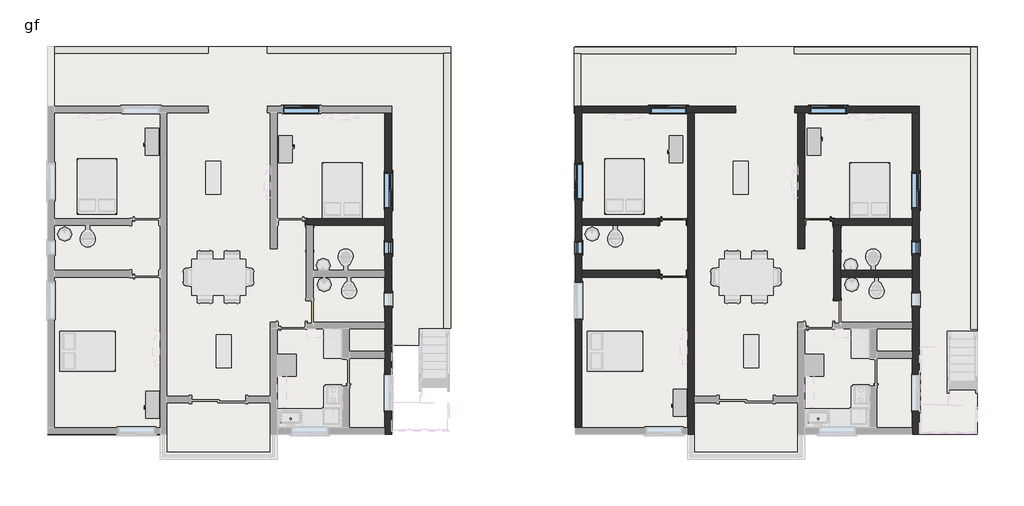
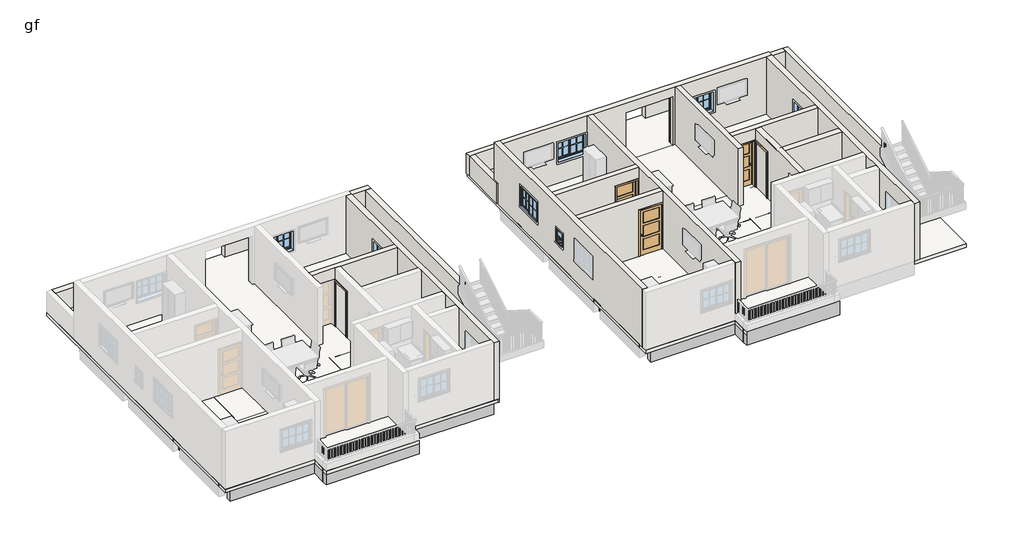
# One storey, part 2 of 8: 20 walls, 14 beams, 9 windows, 5 doors, 2 slabs.
"""IFC4 building model written with IfcOpenShell, lengths in millimetres."""

from ifc_helpers import new_model, si_unit, frame, origin, origin_with_axes, place, context, project, spatial, polyline, outline, extrude, faceted_brep, transform, mapped, element, save
from components import door_2334f446, door_80766924, door_85036156, window_608ea798, window_2eef0573, window_a5b1ea32

model = new_model("IFC4")

# Units and contexts
model_context = context("Model", 3, world=origin())
ifc_project = project(units=[si_unit("LENGTHUNIT", "METRE", prefix="MILLI")], contexts=[model_context])

# Site, building, storey
site = spatial("IfcSite", under=ifc_project)
building = spatial("IfcBuilding", under=site)
storey = spatial("IfcBuildingStorey", under=building, Name="gf", Elevation=609.6)

# Beams
placement = place(None, origin())
element("IfcBeam", 1, ObjectType="Concrete-Rectangular Beam", at=placement, inside=storey, context=model_context, shape_type="SweptSolid", body=[
    extrude(outline(polyline([(-16071.9993763, -4605.3064015), (-16071.9993763, -4376.7064015), (-12490.5993763, -4376.7064015), (-12490.5993763, -4605.3064015), (-16071.9993763, -4605.3064015)])), origin_with_axes(), (0.0, 0.0, 1.0), 609.6),
])
element("IfcBeam", 2, ObjectType="Concrete-Rectangular Beam", at=placement, inside=storey, context=model_context, shape_type="Brep", body=[
    faceted_brep([(-8528.1993763, -5443.5064015, 609.6), (-8528.1993763, -5214.9064015, 609.6), (-8756.7993763, -5214.9064015, 609.6), (-12261.9993763, -5214.9064015, 609.6), (-12490.5993763, -5214.9064015, 609.6), (-12490.5993763, -5443.5064015, 609.6), (-8528.1993763, -5443.5064015, 0.0), (-12490.5993763, -5443.5064015, 0.0), (-8528.1993763, -5214.9064015, 0.0), (-12490.5993763, -5214.9064015, 0.0), (-12261.9993763, -5214.9064015, 0.0), (-8756.7993763, -5214.9064015, 0.0)], [[[0, 1, 2, 3, 4, 5]], [[6, 0, 5, 7]], [[8, 6, 7, 9, 10, 11]], [[1, 8, 11, 10, 9, 4, 3, 2]], [[1, 0, 6, 8]], [[5, 4, 9, 7]]]),
])
element("IfcBeam", 3, ObjectType="Concrete-Rectangular Beam", at=placement, inside=storey, context=model_context, shape_type="Brep", body=[
    faceted_brep([(-8528.1993763, -4376.7064015, 609.6), (-8528.1993763, -4605.3064015, 609.6), (-4870.5993763, -4605.3064015, 609.6), (-4870.5993763, -4376.7064015, 609.6), (-6089.7993763, -4376.7064015, 609.6), (-6318.3993763, -4376.7064015, 609.6), (-8528.1993763, -4376.7064015, 0.0), (-4870.5993763, -4376.7064015, 0.0), (-6089.7993763, -4376.7064015, 0.0), (-6318.3993763, -4376.7064015, 0.0), (-8528.1993763, -4605.3064015, 0.0), (-4870.5993763, -4605.3064015, 0.0)], [[[0, 1, 2, 3, 4, 5]], [[6, 0, 5, 4, 3, 7, 8, 9]], [[10, 6, 9, 8, 7, 11]], [[1, 10, 11, 2]], [[1, 0, 6, 10]], [[3, 2, 11, 7]]]),
])
element("IfcBeam", 4, ObjectType="Concrete-Rectangular Beam", at=placement, inside=storey, context=model_context, shape_type="Brep", body=[
    faceted_brep([(-8528.1993763, -795.3064015, 609.6), (-8528.1993763, -1023.9064015, 609.6), (-6318.3993763, -1023.9064015, 609.6), (-6089.7993763, -1023.9064015, 609.6), (-4870.5993763, -1023.9064015, 609.6), (-4870.5993763, -795.3064015, 609.6), (-7308.9993763, -795.3064015, 609.6), (-7537.5993763, -795.3064015, 609.6), (-8528.1993763, -795.3064015, 0.0), (-4870.5993763, -795.3064015, 0.0), (-7308.9993763, -795.3064015, 0.0), (-7537.5993763, -795.3064015, 0.0), (-8528.1993763, -1023.9064015, 0.0), (-4870.5993763, -1023.9064015, 0.0), (-6089.7993763, -1023.9064015, 0.0), (-6318.3993763, -1023.9064015, 0.0)], [[[0, 1, 2, 3, 4, 5, 6, 7]], [[8, 0, 7, 6, 5, 9, 10, 11]], [[12, 8, 11, 10, 9, 13, 14, 15]], [[1, 12, 15, 14, 13, 4, 3, 2]], [[1, 0, 8, 12]], [[5, 4, 13, 9]]]),
])
element("IfcBeam", 5, ObjectType="Concrete-Rectangular Beam", at=placement, inside=storey, context=model_context, shape_type="Brep", body=[
    faceted_brep([(-6318.3993763, -4376.7064015, 609.6), (-6089.7993763, -4376.7064015, 609.6), (-6089.7993763, -2014.5064015, 609.6), (-6089.7993763, -1785.9064015, 609.6), (-6089.7993763, -1023.9064015, 609.6), (-6318.3993763, -1023.9064015, 609.6), (-6089.7993763, -4376.7064015, 0.0), (-6089.7993763, -2014.5064015, 0.0), (-6089.7993763, -1785.9064015, 0.0), (-6089.7993763, -1023.9064015, 0.0), (-6318.3993763, -4376.7064015, 0.0), (-6318.3993763, -1023.9064015, 0.0)], [[[0, 1, 2, 3, 4, 5]], [[1, 6, 7, 8, 9, 4, 3, 2]], [[6, 10, 11, 9, 8, 7]], [[10, 0, 5, 11]], [[1, 0, 10, 6]], [[5, 4, 9, 11]]]),
])
element("IfcBeam", 6, ObjectType="Concrete-Rectangular Beam", at=placement, inside=storey, context=model_context, shape_type="SweptSolid", body=[
    extrude(outline(polyline([(-4870.5993763, -1785.9064015), (-4870.5993763, -2014.5064015), (-6089.7993763, -2014.5064015), (-6089.7993763, -1785.9064015), (-4870.5993763, -1785.9064015)])), origin_with_axes(), (0.0, 0.0, 1.0), 609.6),
])
element("IfcBeam", 7, ObjectType="Concrete-Rectangular Beam", at=placement, inside=storey, context=model_context, shape_type="Brep", body=[
    faceted_brep([(-8756.7993763, -1023.9064015, 609.6), (-8756.7993763, -795.3064015, 609.6), (-12261.9993763, -795.3064015, 609.6), (-12261.9993763, -1023.9064015, 609.6), (-8756.7993763, -795.3064015, 0.0), (-12261.9993763, -795.3064015, 0.0), (-8756.7993763, -1023.9064015, 0.0), (-12261.9993763, -1023.9064015, 0.0)], [[[0, 1, 2, 3]], [[1, 4, 5, 2]], [[4, 6, 7, 5]], [[6, 0, 3, 7]], [[1, 0, 6, 4]], [[3, 2, 5, 7]]]),
    faceted_brep([(-16071.9993763, -1023.9064015, 609.6), (-16071.9993763, -795.3064015, 609.6), (-16071.9993763, -795.3064015, 0.0), (-16071.9993763, -1023.9064015, 0.0), (-12490.5993763, -795.3064015, 609.6), (-12490.5993763, -1023.9064015, 609.6), (-12490.5993763, -1023.9064015, 0.0), (-12490.5993763, -795.3064015, 0.0), (-13481.1993763, -795.3064015, 609.6), (-13709.7993763, -795.3064015, 609.6), (-13481.1993763, -795.3064015, 0.0), (-13709.7993763, -795.3064015, 0.0)], [[[0, 1, 2, 3]], [[4, 5, 6, 7]], [[1, 0, 5, 4, 8, 9]], [[2, 1, 9, 8, 4, 7, 10, 11]], [[3, 2, 11, 10, 7, 6]], [[0, 3, 6, 5]]]),
])
element("IfcBeam", 8, ObjectType="Concrete-Rectangular Beam", at=placement, inside=storey, context=model_context, shape_type="SweptSolid", body=[
    extrude(outline(polyline([(-12261.9993763, -3538.5064015), (-12261.9993763, -3309.9064015), (-8756.7993763, -3309.9064015), (-8756.7993763, -3538.5064015), (-12261.9993763, -3538.5064015)])), origin_with_axes(), (0.0, 0.0, 1.0), 609.6),
])
element("IfcBeam", 9, ObjectType="Concrete-Rectangular Beam", at=placement, inside=storey, context=model_context, shape_type="SweptSolid", body=[
    extrude(outline(polyline([(1802.5761273, -4605.3064015), (1802.5761273, -4376.7064015), (5383.9761273, -4376.7064015), (5383.9761273, -4605.3064015), (1802.5761273, -4605.3064015)])), origin_with_axes(), (0.0, 0.0, 1.0), 609.6),
])
element("IfcBeam", 10, ObjectType="Concrete-Rectangular Beam", at=placement, inside=storey, context=model_context, shape_type="Brep", body=[
    faceted_brep([(9346.3761273, -5443.5064015, 609.6), (9346.3761273, -5214.9064015, 609.6), (9117.7761273, -5214.9064015, 609.6), (5612.5761273, -5214.9064015, 609.6), (5383.9761273, -5214.9064015, 609.6), (5383.9761273, -5443.5064015, 609.6), (9346.3761273, -5443.5064015, 0.0), (5383.9761273, -5443.5064015, 0.0), (9346.3761273, -5214.9064015, 0.0), (5383.9761273, -5214.9064015, 0.0), (5612.5761273, -5214.9064015, 0.0), (9117.7761273, -5214.9064015, 0.0)], [[[0, 1, 2, 3, 4, 5]], [[6, 0, 5, 7]], [[8, 6, 7, 9, 10, 11]], [[1, 8, 11, 10, 9, 4, 3, 2]], [[1, 0, 6, 8]], [[5, 4, 9, 7]]]),
])
element("IfcBeam", 11, ObjectType="Concrete-Rectangular Beam", at=placement, inside=storey, context=model_context, shape_type="Brep", body=[
    faceted_brep([(9117.7761273, -1023.9064015, 609.6), (9117.7761273, -795.3064015, 609.6), (5612.5761273, -795.3064015, 609.6), (5612.5761273, -1023.9064015, 609.6), (9117.7761273, -795.3064015, 0.0), (5612.5761273, -795.3064015, 0.0), (9117.7761273, -1023.9064015, 0.0), (5612.5761273, -1023.9064015, 0.0)], [[[0, 1, 2, 3]], [[1, 4, 5, 2]], [[4, 6, 7, 5]], [[6, 0, 3, 7]], [[1, 0, 6, 4]], [[3, 2, 5, 7]]]),
    faceted_brep([(1802.5761273, -1023.9064015, 609.6), (1802.5761273, -795.3064015, 609.6), (1802.5761273, -795.3064015, 0.0), (1802.5761273, -1023.9064015, 0.0), (5383.9761273, -795.3064015, 609.6), (5383.9761273, -1023.9064015, 609.6), (5383.9761273, -1023.9064015, 0.0), (5383.9761273, -795.3064015, 0.0), (4393.3761273, -795.3064015, 609.6), (4164.7761273, -795.3064015, 609.6), (4393.3761273, -795.3064015, 0.0), (4164.7761273, -795.3064015, 0.0)], [[[0, 1, 2, 3]], [[4, 5, 6, 7]], [[1, 0, 5, 4, 8, 9]], [[2, 1, 9, 8, 4, 7, 10, 11]], [[3, 2, 11, 10, 7, 6]], [[0, 3, 6, 5]]]),
])
element("IfcBeam", 12, ObjectType="Concrete-Rectangular Beam", at=placement, inside=storey, context=model_context, shape_type="SweptSolid", body=[
    extrude(outline(polyline([(5612.5761273, -3538.5064015), (5612.5761273, -3309.9064015), (9117.7761273, -3309.9064015), (9117.7761273, -3538.5064015), (5612.5761273, -3538.5064015)])), origin_with_axes(), (0.0, 0.0, 1.0), 609.6),
])
element("IfcBeam", 13, ObjectType="Concrete-Rectangular Beam", at=placement, inside=storey, context=model_context, shape_type="SweptSolid", body=[
    extrude(outline(polyline([(-12490.5993763, -4605.3064015), (-12261.9993763, -4605.3064015), (-12261.9993763, -5214.9064015), (-12490.5993763, -5214.9064015), (-12490.5993763, -4605.3064015)])), origin_with_axes(), (0.0, 0.0, 1.0), 609.6),
])
element("IfcBeam", 14, ObjectType="Concrete-Rectangular Beam", at=placement, inside=storey, context=model_context, shape_type="SweptSolid", body=[
    extrude(outline(polyline([(5383.9761273, -4605.3064015), (5612.5761273, -4605.3064015), (5612.5761273, -5214.9064015), (5383.9761273, -5214.9064015), (5383.9761273, -4605.3064015)])), origin_with_axes(), (0.0, 0.0, 1.0), 609.6),
])

# Doors
door_shape = door_2334f446(model_context)
element("IfcDoor", 15, ObjectType="Door-Interior-Single-3_Panel_Vert-Wood : 36\" x 80\"", at=placement, inside=storey, context=model_context, shape_type="MappedRepresentation", body=[
    mapped(door_shape, transform((4888.6761273, 2598.7685985, 609.6), x_axis=(1.0, 0.0, 0.0), y_axis=(0.0, 1.0, 0.0), z_axis=(0.0, 0.0, 1.0))),
])
door_2_shape = door_80766924(model_context)
element("IfcDoor", 16, ObjectType="Door-Interior-Single-3_Panel_Vert-Wood : 36\" x 80\"", at=placement, inside=storey, context=model_context, shape_type="MappedRepresentation", body=[
    mapped(door_2_shape, transform((4888.6761273, 839.8185985, 609.6), x_axis=(1.0, 0.0, 0.0), y_axis=(0.0, 1.0, 0.0), z_axis=(0.0, 0.0, 1.0))),
])
element("IfcDoor", 17, ObjectType="Door-Interior-Single-3_Panel_Vert-Wood : 36\" x 80\"", at=placement, inside=storey, context=model_context, shape_type="MappedRepresentation", body=[
    mapped(door_2_shape, transform((9841.6761273, 2598.7685985, 609.6), x_axis=(-1.0, 0.0, 0.0), y_axis=(0.0, -1.0, 0.0), z_axis=(0.0, 0.0, 1.0))),
])
door_3_shape = door_85036156(model_context)
element("IfcDoor", 18, ObjectType="Single-Flush : 30\" x 80\"", at=placement, inside=storey, context=model_context, shape_type="MappedRepresentation", body=[
    mapped(door_3_shape, transform((-7423.2993763, 2024.0935985, 609.6), x_axis=(0.0, 1.0, 0.0), y_axis=(-1.0, 0.0, 0.0), z_axis=(0.0, 0.0, 1.0))),
])
element("IfcDoor", 19, ObjectType="Single-Flush : 30\" x 80\"", at=placement, inside=storey, context=model_context, shape_type="MappedRepresentation", body=[
    mapped(door_3_shape, transform((10451.2761273, 2024.0935985, 609.6), x_axis=(0.0, 1.0, 0.0), y_axis=(-1.0, 0.0, 0.0), z_axis=(0.0, 0.0, 1.0))),
])

# Slabs
element("IfcSlab", 20, at=placement, inside=storey, context=model_context, shape_type="SweptSolid", body=[
    extrude(outline(polyline([(15201.0761273, 8539.1935985), (15201.0761273, -4598.9564015), (9346.3761273, -4598.9564015), (9346.3761273, -5437.1564015), (5383.9761273, -5437.1564015), (5383.9761273, -4605.3064015), (1573.9761273, -4605.3064015), (1573.9761273, 8539.1935985), (15201.0761273, 8539.1935985)])), frame((0.0, 0.0, 457.2), z_axis=(0.0, 0.0, 1.0), x_axis=(1.0, 0.0, 0.0)), (0.0, 0.0, 1.0), 152.4),
])
element("IfcSlab", 21, at=placement, inside=storey, context=model_context, shape_type="SweptSolid", body=[
    extrude(outline(polyline([(-2647.3594779, 8539.1935985), (-2647.3594779, -998.5064015), (-3676.7993763, -998.5064015), (-3676.7993763, -1582.7064015), (-4641.9993763, -1582.7064015), (-4641.9993763, -4605.3064015), (-4692.7993763, -4605.3064015), (-8528.1993763, -4605.3064015), (-8528.1993763, -5443.5064015), (-12490.5993763, -5443.5064015), (-12490.5993763, -4611.6564015), (-16300.5993763, -4611.6564015), (-16300.5993763, 8539.1935985), (-2647.3594779, 8539.1935985)])), frame((0.0, 0.0, 457.2), z_axis=(0.0, 0.0, 1.0), x_axis=(1.0, 0.0, 0.0)), (0.0, 0.0, 1.0), 152.4),
])

# Walls
element("IfcWall", 22, at=placement, inside=storey, context=model_context, shape_type="Brep", body=[
    faceted_brep([(-4870.5993763, 6291.2935985, 609.6), (-4870.5993763, 2709.8935985, 609.6), (-4870.5993763, 2481.2935985, 609.6), (-4870.5993763, 957.2935985, 609.6), (-4870.5993763, 728.6935985, 609.6), (-4870.5993763, -795.3064015, 609.6), (-4870.5993763, -1023.9064015, 609.6), (-4870.5993763, -1785.9064015, 609.6), (-4870.5993763, -2014.5064015, 609.6), (-4870.5993763, -4376.7064015, 609.6), (-4870.5993763, -4605.3064015, 609.6), (-4870.5993763, -4605.3064015, 3200.4), (-4870.5993763, -4376.7064015, 3200.4), (-4870.5993763, -2014.5064015, 3200.4), (-4870.5993763, -1785.9064015, 3200.4), (-4870.5993763, -1023.9064015, 3200.4), (-4870.5993763, -795.3064015, 3200.4), (-4870.5993763, 728.6935985, 3200.4), (-4870.5993763, 957.2935985, 3200.4), (-4870.5993763, 2481.2935985, 3200.4), (-4870.5993763, 2709.8935985, 3200.4), (-4870.5993763, 6291.2935985, 3200.4), (-4870.5993763, 4271.9935985, 2438.4), (-4870.5993763, 3052.7935985, 2438.4), (-4870.5993763, 3052.7935985, 1524.0), (-4870.5993763, 4271.9935985, 1524.0), (-4870.5993763, -249.2064015, 2133.6), (-4870.5993763, -249.2064015, 1524.0), (-4870.5993763, 182.5935985, 1524.0), (-4870.5993763, 182.5935985, 2133.6), (-4870.5993763, 1503.3935985, 2133.6), (-4870.5993763, 1503.3935985, 1524.0), (-4870.5993763, 1935.1935985, 1524.0), (-4870.5993763, 1935.1935985, 2133.6), (-4870.5993763, -3805.2064015, 2438.4), (-4870.5993763, -3805.2064015, 1524.0), (-4870.5993763, -2586.0064015, 1524.0), (-4870.5993763, -2586.0064015, 2438.4), (-4641.9993763, 6291.2935985, 609.6), (-4641.9993763, 6291.2935985, 3200.4), (-4641.9993763, -4605.3064015, 3200.4), (-4641.9993763, -4605.3064015, 609.6), (-4641.9993763, 4271.9935985, 2438.4), (-4641.9993763, 4271.9935985, 1524.0), (-4641.9993763, 3052.7935985, 1524.0), (-4641.9993763, 3052.7935985, 2438.4), (-4641.9993763, -249.2064015, 2133.6), (-4641.9993763, 182.5935985, 2133.6), (-4641.9993763, 182.5935985, 1524.0), (-4641.9993763, -249.2064015, 1524.0), (-4641.9993763, 1503.3935985, 2133.6), (-4641.9993763, 1935.1935985, 2133.6), (-4641.9993763, 1935.1935985, 1524.0), (-4641.9993763, 1503.3935985, 1524.0), (-4641.9993763, -3805.2064015, 2438.4), (-4641.9993763, -2586.0064015, 2438.4), (-4641.9993763, -2586.0064015, 1524.0), (-4641.9993763, -3805.2064015, 1524.0)], [[[0, 1, 2, 3, 4, 5, 6, 7, 8, 9, 10, 11, 12, 13, 14, 15, 16, 17, 18, 19, 20, 21], [22, 23, 24, 25], [26, 27, 28, 29], [30, 31, 32, 33], [34, 35, 36, 37]], [[38, 39, 40, 41], [42, 43, 44, 45], [46, 47, 48, 49], [50, 51, 52, 53], [54, 55, 56, 57]], [[10, 9, 8, 7, 6, 5, 4, 3, 2, 1, 0, 38, 41]], [[21, 20, 19, 18, 17, 16, 15, 14, 13, 12, 11, 40, 39]], [[0, 21, 39, 38]], [[11, 10, 41, 40]], [[43, 42, 22, 25]], [[44, 43, 25, 24]], [[45, 44, 24, 23]], [[42, 45, 23, 22]], [[27, 26, 46, 49]], [[28, 27, 49, 48]], [[29, 28, 48, 47]], [[26, 29, 47, 46]], [[31, 30, 50, 53]], [[32, 31, 53, 52]], [[33, 32, 52, 51]], [[30, 33, 51, 50]], [[35, 34, 54, 57]], [[36, 35, 57, 56]], [[37, 36, 56, 55]], [[34, 37, 55, 54]]]),
])
element("IfcWall", 23, at=placement, inside=storey, context=model_context, shape_type="Brep", body=[
    faceted_brep([(-4870.5993763, 2481.2935985, 3200.4), (-7308.9993763, 2481.2935985, 3200.4), (-7537.5993763, 2481.2935985, 3200.4), (-8528.1993763, 2481.2935985, 3200.4), (-8528.1993763, 2481.2935985, 609.6), (-8515.4993763, 2481.2935985, 609.6), (-8515.4993763, 2481.2935985, 2667.0), (-7550.2993763, 2481.2935985, 2667.0), (-7550.2993763, 2481.2935985, 609.6), (-7537.5993763, 2481.2935985, 609.6), (-7308.9993763, 2481.2935985, 609.6), (-4870.5993763, 2481.2935985, 609.6), (-8528.1993763, 2709.8935985, 3200.4), (-4870.5993763, 2709.8935985, 3200.4), (-4870.5993763, 2709.8935985, 609.6), (-7550.2993763, 2709.8935985, 609.6), (-7550.2993763, 2709.8935985, 2667.0), (-8515.4993763, 2709.8935985, 2667.0), (-8515.4993763, 2709.8935985, 609.6), (-8528.1993763, 2709.8935985, 609.6)], [[[0, 1, 2, 3, 4, 5, 6, 7, 8, 9, 10, 11]], [[12, 13, 14, 15, 16, 17, 18, 19]], [[14, 11, 10, 9, 8, 15]], [[4, 19, 18, 5]], [[3, 2, 1, 0, 13, 12]], [[0, 11, 14, 13]], [[17, 6, 5, 18]], [[6, 17, 16, 7]], [[7, 16, 15, 8]], [[4, 3, 12, 19]]]),
])
element("IfcWall", 24, at=placement, inside=storey, context=model_context, shape_type="Brep", body=[
    faceted_brep([(1573.9761273, 6519.8935985, 609.6), (1573.9761273, -4376.7064015, 609.6), (1573.9761273, -4376.7064015, 3200.4), (1573.9761273, 6519.8935985, 3200.4), (1573.9761273, 4576.7935985, 2438.4), (1573.9761273, 3357.5935985, 2438.4), (1573.9761273, 3357.5935985, 1524.0), (1573.9761273, 4576.7935985, 1524.0), (1573.9761273, -681.0064015, 2438.4), (1573.9761273, -681.0064015, 1524.0), (1573.9761273, 538.1935985, 1524.0), (1573.9761273, 538.1935985, 2438.4), (1573.9761273, 1935.1935985, 2133.6), (1573.9761273, 1503.3935985, 2133.6), (1573.9761273, 1503.3935985, 1524.0), (1573.9761273, 1935.1935985, 1524.0), (1802.5761273, 6519.8935985, 609.6), (1802.5761273, 6519.8935985, 3200.4), (1802.5761273, 6291.2935985, 3200.4), (1802.5761273, 2709.8935985, 3200.4), (1802.5761273, 2481.2935985, 3200.4), (1802.5761273, 957.2935985, 3200.4), (1802.5761273, 728.6935985, 3200.4), (1802.5761273, -4376.7064015, 3200.4), (1802.5761273, -4376.7064015, 609.6), (1802.5761273, 728.6935985, 609.6), (1802.5761273, 957.2935985, 609.6), (1802.5761273, 2481.2935985, 609.6), (1802.5761273, 2709.8935985, 609.6), (1802.5761273, 6291.2935985, 609.6), (1802.5761273, 4576.7935985, 2438.4), (1802.5761273, 4576.7935985, 1524.0), (1802.5761273, 3357.5935985, 1524.0), (1802.5761273, 3357.5935985, 2438.4), (1802.5761273, -681.0064015, 2438.4), (1802.5761273, 538.1935985, 2438.4), (1802.5761273, 538.1935985, 1524.0), (1802.5761273, -681.0064015, 1524.0), (1802.5761273, 1935.1935985, 2133.6), (1802.5761273, 1935.1935985, 1524.0), (1802.5761273, 1503.3935985, 1524.0), (1802.5761273, 1503.3935985, 2133.6)], [[[0, 1, 2, 3], [4, 5, 6, 7], [8, 9, 10, 11], [12, 13, 14, 15]], [[16, 17, 18, 19, 20, 21, 22, 23, 24, 25, 26, 27, 28, 29], [30, 31, 32, 33], [34, 35, 36, 37], [38, 39, 40, 41]], [[1, 0, 16, 29, 28, 27, 26, 25, 24]], [[3, 2, 23, 22, 21, 20, 19, 18, 17]], [[0, 3, 17, 16]], [[2, 1, 24, 23]], [[31, 30, 4, 7]], [[32, 31, 7, 6]], [[33, 32, 6, 5]], [[30, 33, 5, 4]], [[9, 8, 34, 37]], [[10, 9, 37, 36]], [[11, 10, 36, 35]], [[8, 11, 35, 34]], [[39, 38, 12, 15]], [[40, 39, 15, 14]], [[41, 40, 14, 13]], [[38, 41, 13, 12]]]),
])
element("IfcWall", 25, at=placement, inside=storey, context=model_context, shape_type="SweptSolid", body=[
    extrude(outline(polyline([(3200.4, 5383.9761273), (3200.4, 1802.5761273), (609.6, 1802.5761273), (609.6, 4406.0761273), (2667.0, 4406.0761273), (2667.0, 5371.2761273), (609.6, 5371.2761273), (609.6, 5383.9761273), (3200.4, 5383.9761273)])), frame((0.0, 2481.2935985, 0.0), z_axis=(0.0, 1.0, 0.0), x_axis=(0.0, 0.0, 1.0)), (0.0, 0.0, 1.0), 228.6),
])
element("IfcWall", 26, at=placement, inside=storey, context=model_context, shape_type="Brep", body=[
    faceted_brep([(13232.5761273, 6291.2935985, 3200.4), (13003.9761273, 6291.2935985, 3200.4), (9346.3761273, 6291.2935985, 3200.4), (9117.7761273, 6291.2935985, 3200.4), (5612.5761273, 6291.2935985, 3200.4), (5383.9761273, 6291.2935985, 3200.4), (1802.5761273, 6291.2935985, 3200.4), (1802.5761273, 6291.2935985, 609.6), (5383.9761273, 6291.2935985, 609.6), (5612.5761273, 6291.2935985, 609.6), (7012.8761273, 6291.2935985, 609.6), (7012.8761273, 6291.2935985, 2779.1), (9012.8761273, 6291.2935985, 2779.1), (9012.8761273, 6291.2935985, 609.6), (9117.7761273, 6291.2935985, 609.6), (9346.3761273, 6291.2935985, 609.6), (13003.9761273, 6291.2935985, 609.6), (13232.5761273, 6291.2935985, 609.6), (9536.8761273, 6291.2935985, 2438.4), (10756.0761273, 6291.2935985, 2438.4), (10756.0761273, 6291.2935985, 1524.0), (9536.8761273, 6291.2935985, 1524.0), (5345.8761273, 6291.2935985, 2438.4), (5345.8761273, 6291.2935985, 1524.0), (4126.6761273, 6291.2935985, 1524.0), (4126.6761273, 6291.2935985, 2438.4), (1802.5761273, 6519.8935985, 3200.4), (13232.5761273, 6519.8935985, 3200.4), (13232.5761273, 6519.8935985, 609.6), (9012.8761273, 6519.8935985, 609.6), (9012.8761273, 6519.8935985, 2779.1), (7012.8761273, 6519.8935985, 2779.1), (7012.8761273, 6519.8935985, 609.6), (1802.5761273, 6519.8935985, 609.6), (9536.8761273, 6519.8935985, 2438.4), (9536.8761273, 6519.8935985, 1524.0), (10756.0761273, 6519.8935985, 1524.0), (10756.0761273, 6519.8935985, 2438.4), (5345.8761273, 6519.8935985, 2438.4), (4126.6761273, 6519.8935985, 2438.4), (4126.6761273, 6519.8935985, 1524.0), (5345.8761273, 6519.8935985, 1524.0), (7012.8761273, 6499.8935985, 609.6), (6997.8761273, 6499.8935985, 609.6), (6997.8761273, 6429.8935985, 609.6), (7012.8761273, 6429.8935985, 609.6), (9012.8761273, 6429.8935985, 609.6), (9027.8761273, 6429.8935985, 609.6), (9027.8761273, 6499.8935985, 609.6), (9012.8761273, 6499.8935985, 609.6), (9012.8761273, 6499.8935985, 2779.1), (7012.8761273, 6499.8935985, 2779.1), (7012.8761273, 6429.8935985, 2779.1), (9012.8761273, 6429.8935985, 2779.1), (6997.8761273, 6429.8935985, 2794.1), (9027.8761273, 6429.8935985, 2794.1), (9027.8761273, 6499.8935985, 2794.1), (6997.8761273, 6499.8935985, 2794.1)], [[[0, 1, 2, 3, 4, 5, 6, 7, 8, 9, 10, 11, 12, 13, 14, 15, 16, 17], [18, 19, 20, 21], [22, 23, 24, 25]], [[26, 27, 28, 29, 30, 31, 32, 33], [34, 35, 36, 37], [38, 39, 40, 41]], [[7, 33, 32, 42, 43, 44, 45, 10, 9, 8]], [[28, 17, 16, 15, 14, 13, 46, 47, 48, 49, 29]], [[6, 5, 4, 3, 2, 1, 0, 27, 26]], [[7, 6, 26, 33]], [[0, 17, 28, 27]], [[50, 51, 31, 30]], [[52, 53, 12, 11]], [[45, 52, 11, 10]], [[53, 46, 13, 12]], [[53, 52, 45, 44, 54, 55, 47, 46]], [[47, 55, 56, 48]], [[51, 50, 49, 48, 56, 57, 43, 42]], [[49, 50, 30, 29]], [[51, 42, 32, 31]], [[54, 44, 43, 57]], [[55, 54, 57, 56]], [[35, 34, 18, 21]], [[36, 35, 21, 20]], [[37, 36, 20, 19]], [[34, 37, 19, 18]], [[23, 22, 38, 41]], [[24, 23, 41, 40]], [[25, 24, 40, 39]], [[22, 25, 39, 38]]]),
])
element("IfcWall", 27, at=placement, inside=storey, context=model_context, shape_type="Brep", body=[
    faceted_brep([(13003.9761273, 6291.2935985, 609.6), (13003.9761273, 2709.8935985, 609.6), (13003.9761273, 2481.2935985, 609.6), (13003.9761273, 957.2935985, 609.6), (13003.9761273, 728.6935985, 609.6), (13003.9761273, -795.3064015, 609.6), (13003.9761273, -1023.9064015, 609.6), (13003.9761273, -1785.9064015, 609.6), (13003.9761273, -2014.5064015, 609.6), (13003.9761273, -4376.7064015, 609.6), (13003.9761273, -4605.3064015, 609.6), (13003.9761273, -4605.3064015, 3200.4), (13003.9761273, -4376.7064015, 3200.4), (13003.9761273, -2014.5064015, 3200.4), (13003.9761273, -1785.9064015, 3200.4), (13003.9761273, -1023.9064015, 3200.4), (13003.9761273, -795.3064015, 3200.4), (13003.9761273, 728.6935985, 3200.4), (13003.9761273, 957.2935985, 3200.4), (13003.9761273, 2481.2935985, 3200.4), (13003.9761273, 2709.8935985, 3200.4), (13003.9761273, 6291.2935985, 3200.4), (13003.9761273, 4271.9935985, 2438.4), (13003.9761273, 3052.7935985, 2438.4), (13003.9761273, 3052.7935985, 1524.0), (13003.9761273, 4271.9935985, 1524.0), (13003.9761273, -249.2064015, 2133.6), (13003.9761273, -249.2064015, 1524.0), (13003.9761273, 182.5935985, 1524.0), (13003.9761273, 182.5935985, 2133.6), (13003.9761273, 1503.3935985, 2133.6), (13003.9761273, 1503.3935985, 1524.0), (13003.9761273, 1935.1935985, 1524.0), (13003.9761273, 1935.1935985, 2133.6), (13003.9761273, -3805.2064015, 2438.4), (13003.9761273, -3805.2064015, 1524.0), (13003.9761273, -2586.0064015, 1524.0), (13003.9761273, -2586.0064015, 2438.4), (13232.5761273, 6291.2935985, 609.6), (13232.5761273, 6291.2935985, 3200.4), (13232.5761273, -4605.3064015, 3200.4), (13232.5761273, -4605.3064015, 609.6), (13232.5761273, 4271.9935985, 2438.4), (13232.5761273, 4271.9935985, 1524.0), (13232.5761273, 3052.7935985, 1524.0), (13232.5761273, 3052.7935985, 2438.4), (13232.5761273, -249.2064015, 2133.6), (13232.5761273, 182.5935985, 2133.6), (13232.5761273, 182.5935985, 1524.0), (13232.5761273, -249.2064015, 1524.0), (13232.5761273, 1503.3935985, 2133.6), (13232.5761273, 1935.1935985, 2133.6), (13232.5761273, 1935.1935985, 1524.0), (13232.5761273, 1503.3935985, 1524.0), (13232.5761273, -3805.2064015, 2438.4), (13232.5761273, -2586.0064015, 2438.4), (13232.5761273, -2586.0064015, 1524.0), (13232.5761273, -3805.2064015, 1524.0)], [[[0, 1, 2, 3, 4, 5, 6, 7, 8, 9, 10, 11, 12, 13, 14, 15, 16, 17, 18, 19, 20, 21], [22, 23, 24, 25], [26, 27, 28, 29], [30, 31, 32, 33], [34, 35, 36, 37]], [[38, 39, 40, 41], [42, 43, 44, 45], [46, 47, 48, 49], [50, 51, 52, 53], [54, 55, 56, 57]], [[10, 9, 8, 7, 6, 5, 4, 3, 2, 1, 0, 38, 41]], [[21, 20, 19, 18, 17, 16, 15, 14, 13, 12, 11, 40, 39]], [[0, 21, 39, 38]], [[43, 42, 22, 25]], [[44, 43, 25, 24]], [[45, 44, 24, 23]], [[42, 45, 23, 22]], [[27, 26, 46, 49]], [[28, 27, 49, 48]], [[29, 28, 48, 47]], [[26, 29, 47, 46]], [[31, 30, 50, 53]], [[32, 31, 53, 52]], [[33, 32, 52, 51]], [[30, 33, 51, 50]], [[35, 34, 54, 57]], [[36, 35, 57, 56]], [[37, 36, 56, 55]], [[34, 37, 55, 54]], [[11, 10, 41, 40]]]),
])
element("IfcWall", 28, at=placement, inside=storey, context=model_context, shape_type="Brep", body=[
    faceted_brep([(9117.7761273, 6291.2935985, 609.6), (9117.7761273, 1681.1935985, 609.6), (9117.7761273, 1681.1935985, 3200.4), (9117.7761273, 6291.2935985, 3200.4), (9346.3761273, 6291.2935985, 609.6), (9346.3761273, 6291.2935985, 3200.4), (9346.3761273, 2709.8935985, 3200.4), (9346.3761273, 2481.2935985, 3200.4), (9346.3761273, 1681.1935985, 3200.4), (9346.3761273, 1681.1935985, 609.6), (9346.3761273, 2481.2935985, 609.6), (9346.3761273, 2709.8935985, 609.6)], [[[0, 1, 2, 3]], [[4, 5, 6, 7, 8, 9, 10, 11]], [[1, 0, 4, 11, 10, 9]], [[2, 1, 9, 8]], [[3, 2, 8, 7, 6, 5]], [[0, 3, 5, 4]]]),
])
element("IfcWall", 29, at=placement, inside=storey, context=model_context, shape_type="SweptSolid", body=[
    extrude(outline(polyline([(10565.5761273, 957.2935985), (13003.9761273, 957.2935985), (13003.9761273, 728.6935985), (10565.5761273, 728.6935985), (10565.5761273, 957.2935985)])), frame((0.0, 0.0, 609.6), z_axis=(0.0, 0.0, 1.0), x_axis=(1.0, 0.0, 0.0)), (0.0, 0.0, 1.0), 2590.8),
])
element("IfcWall", 30, at=placement, inside=storey, context=model_context, shape_type="Brep", body=[
    faceted_brep([(10565.5761273, 2481.2935985, 3200.4), (10565.5761273, 957.2935985, 3200.4), (10565.5761273, 728.6935985, 3200.4), (10565.5761273, -795.3064015, 3200.4), (10565.5761273, -795.3064015, 2641.6), (10565.5761273, -71.4064015, 2641.6), (10565.5761273, -71.4064015, 609.6), (10565.5761273, 728.6935985, 609.6), (10565.5761273, 957.2935985, 609.6), (10565.5761273, 2481.2935985, 609.6), (10336.9761273, -795.3064015, 3200.4), (10336.9761273, 2481.2935985, 3200.4), (10336.9761273, 2481.2935985, 609.6), (10336.9761273, -71.4064015, 609.6), (10336.9761273, -71.4064015, 2641.6), (10336.9761273, -795.3064015, 2641.6)], [[[0, 1, 2, 3, 4, 5, 6, 7, 8, 9]], [[10, 11, 12, 13, 14, 15]], [[12, 9, 8, 7, 6, 13]], [[3, 2, 1, 0, 11, 10]], [[3, 10, 15, 4]], [[0, 9, 12, 11]], [[14, 5, 4, 15]], [[5, 14, 13, 6]]]),
])
element("IfcWall", 31, at=placement, inside=storey, context=model_context, shape_type="SweptSolid", body=[
    extrude(outline(polyline([(2481.2935985, 609.6), (2405.0935985, 609.6), (2405.0935985, 2641.6), (1643.0935985, 2641.6), (1643.0935985, 609.6), (957.2935985, 609.6), (957.2935985, 3200.4), (2481.2935985, 3200.4), (2481.2935985, 609.6)])), frame((10336.9761273, 0.0, 0.0), z_axis=(1.0, 0.0, 0.0), x_axis=(0.0, 1.0, 0.0)), (0.0, 0.0, 1.0), 228.6),
])
element("IfcWall", 32, at=placement, inside=storey, context=model_context, shape_type="Brep", body=[
    faceted_brep([(13003.9761273, 2481.2935985, 3200.4), (10565.5761273, 2481.2935985, 3200.4), (10336.9761273, 2481.2935985, 3200.4), (9346.3761273, 2481.2935985, 3200.4), (9346.3761273, 2481.2935985, 609.6), (9359.0761273, 2481.2935985, 609.6), (9359.0761273, 2481.2935985, 2667.0), (10324.2761273, 2481.2935985, 2667.0), (10324.2761273, 2481.2935985, 609.6), (10336.9761273, 2481.2935985, 609.6), (10565.5761273, 2481.2935985, 609.6), (13003.9761273, 2481.2935985, 609.6), (9346.3761273, 2709.8935985, 3200.4), (13003.9761273, 2709.8935985, 3200.4), (13003.9761273, 2709.8935985, 609.6), (10324.2761273, 2709.8935985, 609.6), (10324.2761273, 2709.8935985, 2667.0), (9359.0761273, 2709.8935985, 2667.0), (9359.0761273, 2709.8935985, 609.6), (9346.3761273, 2709.8935985, 609.6)], [[[0, 1, 2, 3, 4, 5, 6, 7, 8, 9, 10, 11]], [[12, 13, 14, 15, 16, 17, 18, 19]], [[14, 11, 10, 9, 8, 15]], [[4, 19, 18, 5]], [[3, 2, 1, 0, 13, 12]], [[0, 11, 14, 13]], [[17, 6, 5, 18]], [[6, 17, 16, 7]], [[7, 16, 15, 8]], [[4, 3, 12, 19]]]),
])
element("IfcWall", 33, at=placement, inside=storey, context=model_context, shape_type="SweptSolid", body=[
    extrude(outline(polyline([(3200.4, 5383.9761273), (3200.4, 1802.5761273), (609.6, 1802.5761273), (609.6, 4406.0761273), (2667.0, 4406.0761273), (2667.0, 5371.2761273), (609.6, 5371.2761273), (609.6, 5383.9761273), (3200.4, 5383.9761273)])), frame((0.0, 728.6935985, 0.0), z_axis=(0.0, 1.0, 0.0), x_axis=(0.0, 0.0, 1.0)), (0.0, 0.0, 1.0), 228.6),
])
element("IfcWall", 34, at=placement, inside=storey, context=model_context, shape_type="Brep", body=[
    faceted_brep([(5612.5761273, -4605.3064015, 609.6), (5612.5761273, -3538.5064015, 609.6), (5612.5761273, -3309.9064015, 609.6), (5612.5761273, 6291.2935985, 609.6), (5612.5761273, 6291.2935985, 3200.4), (5612.5761273, -3309.9064015, 3200.4), (5612.5761273, -3538.5064015, 3200.4), (5612.5761273, -4605.3064015, 3200.4), (5383.9761273, -4605.3064015, 609.6), (5383.9761273, -4605.3064015, 3200.4), (5383.9761273, -4376.7064015, 3200.4), (5383.9761273, 728.6935985, 3200.4), (5383.9761273, 957.2935985, 3200.4), (5383.9761273, 2481.2935985, 3200.4), (5383.9761273, 2709.8935985, 3200.4), (5383.9761273, 6291.2935985, 3200.4), (5383.9761273, 6291.2935985, 609.6), (5383.9761273, 2709.8935985, 609.6), (5383.9761273, 2481.2935985, 609.6), (5383.9761273, 957.2935985, 609.6), (5383.9761273, 728.6935985, 609.6), (5383.9761273, -4376.7064015, 609.6)], [[[0, 1, 2, 3, 4, 5, 6, 7]], [[8, 9, 10, 11, 12, 13, 14, 15, 16, 17, 18, 19, 20, 21]], [[3, 2, 1, 0, 8, 21, 20, 19, 18, 17, 16]], [[7, 6, 5, 4, 15, 14, 13, 12, 11, 10, 9]], [[4, 3, 16, 15]], [[0, 7, 9, 8]]]),
])
element("IfcWall", 35, at=placement, inside=storey, context=model_context, shape_type="Brep", body=[
    faceted_brep([(15204.9910257, -1042.9564015, 609.6), (15204.9910257, 8523.3185985, 609.6), (15204.9910257, 8523.3185985, 1524.0), (15204.9910257, -1042.9564015, 1524.0), (14976.3910257, -1042.9564015, 609.6), (14976.3910257, -1042.9564015, 1524.0), (14976.3910257, 8294.7185985, 1524.0), (14976.3910257, 8523.3185985, 1524.0), (14976.3910257, 8523.3185985, 609.6), (14976.3910257, 8294.7185985, 609.6)], [[[0, 1, 2, 3]], [[4, 5, 6, 7, 8, 9]], [[1, 0, 4, 9, 8]], [[3, 2, 7, 6, 5]], [[0, 3, 5, 4]], [[2, 1, 8, 7]]]),
])
element("IfcWall", 36, at=placement, inside=storey, context=model_context, shape_type="SweptSolid", body=[
    extrude(outline(polyline([(9003.4761273, 8523.3185985), (14976.3910257, 8523.3185985), (14976.3910257, 8294.7185985), (9003.4761273, 8294.7185985), (9003.4761273, 8523.3185985)])), frame((0.0, 0.0, 609.6), z_axis=(0.0, 0.0, 1.0), x_axis=(1.0, 0.0, 0.0)), (0.0, 0.0, 1.0), 914.4),
])
element("IfcWall", 37, at=placement, inside=storey, context=model_context, shape_type="SweptSolid", body=[
    extrude(outline(polyline([(1539.7910257, 6275.4185985), (1539.7910257, 8294.7185985), (1768.3910257, 8294.7185985), (1768.3910257, 6275.4185985), (1539.7910257, 6275.4185985)])), frame((0.0, 0.0, 609.6), z_axis=(0.0, 0.0, 1.0), x_axis=(1.0, 0.0, 0.0)), (0.0, 0.0, 1.0), 914.4),
])
element("IfcWall", 38, at=placement, inside=storey, context=model_context, shape_type="SweptSolid", body=[
    extrude(outline(polyline([(-10852.2993763, 8310.5935985), (-16071.9993763, 8310.5935985), (-16071.9993763, 8539.1935985), (-10852.2993763, 8539.1935985), (-10852.2993763, 8310.5935985)])), frame((0.0, 0.0, 609.6), z_axis=(0.0, 0.0, 1.0), x_axis=(1.0, 0.0, 0.0)), (0.0, 0.0, 1.0), 914.4),
])
element("IfcWall", 39, at=placement, inside=storey, context=model_context, shape_type="SweptSolid", body=[
    extrude(outline(polyline([(-2875.9594779, -998.5064015), (-2875.9594779, 8310.5935985), (-2647.3594779, 8310.5935985), (-2647.3594779, -998.5064015), (-2875.9594779, -998.5064015)])), frame((0.0, 0.0, 609.6), z_axis=(0.0, 0.0, 1.0), x_axis=(1.0, 0.0, 0.0)), (0.0, 0.0, 1.0), 914.4),
])
element("IfcWall", 40, at=placement, inside=storey, context=model_context, shape_type="Brep", body=[
    faceted_brep([(7012.8761273, 8523.3185985, 609.6), (1539.7910257, 8523.3185985, 609.6), (1539.7910257, 8523.3185985, 1524.0), (7012.8761273, 8523.3185985, 1524.0), (7012.8761273, 8294.7185985, 609.6), (7012.8761273, 8294.7185985, 1524.0), (1768.3910257, 8294.7185985, 1524.0), (1539.7910257, 8294.7185985, 1524.0), (1539.7910257, 8294.7185985, 609.6), (1768.3910257, 8294.7185985, 609.6)], [[[0, 1, 2, 3]], [[4, 5, 6, 7, 8, 9]], [[1, 0, 4, 9, 8]], [[3, 2, 7, 6, 5]], [[0, 3, 5, 4]], [[2, 1, 8, 7]]]),
])
element("IfcWall", 41, at=placement, inside=storey, context=model_context, shape_type="Brep", body=[
    faceted_brep([(-8861.6993763, 8310.5935985, 609.6), (-2875.9594779, 8310.5935985, 609.6), (-2647.3594779, 8310.5935985, 609.6), (-2647.3594779, 8310.5935985, 1524.0), (-2875.9594779, 8310.5935985, 1524.0), (-8861.6993763, 8310.5935985, 1524.0), (-8861.6993763, 8539.1935985, 609.6), (-8861.6993763, 8539.1935985, 1524.0), (-2647.3594779, 8539.1935985, 1524.0), (-2647.3594779, 8539.1935985, 609.6)], [[[0, 1, 2, 3, 4, 5]], [[6, 7, 8, 9]], [[2, 1, 0, 6, 9]], [[5, 4, 3, 8, 7]], [[0, 5, 7, 6]], [[3, 2, 9, 8]]]),
])

# Windows
window_shape = window_608ea798(model_context)
element("IfcWindow", 42, ObjectType="Window-Fixed-Transom : 17\" x 24\"", at=placement, inside=storey, context=model_context, shape_type="MappedRepresentation", body=[
    mapped(window_shape, transform((-4756.2993763, 1719.2935985, 609.6), x_axis=(0.0, -1.0, 0.0), y_axis=(1.0, 0.0, 0.0), z_axis=(0.0, 0.0, 1.0))),
])
element("IfcWindow", 43, ObjectType="Window-Fixed-Transom : 17\" x 24\"", at=placement, inside=storey, context=model_context, shape_type="MappedRepresentation", body=[
    mapped(window_shape, transform((13118.2761273, 1719.2935985, 609.6), x_axis=(0.0, -1.0, 0.0), y_axis=(1.0, 0.0, 0.0), z_axis=(0.0, 0.0, 1.0))),
])
element("IfcWindow", 44, ObjectType="Window-Fixed-Transom : 17\" x 24\"", at=placement, inside=storey, context=model_context, shape_type="MappedRepresentation", body=[
    mapped(window_shape, transform((1688.2761273, 1719.2935985, 609.6), x_axis=(0.0, 1.0, 0.0), y_axis=(-1.0, 0.0, 0.0), z_axis=(0.0, 0.0, 1.0))),
])
window_2_shape = window_2eef0573(model_context)
element("IfcWindow", 45, ObjectType="Window-Sliding-Double : 48\" x 36\"", at=placement, inside=storey, context=model_context, shape_type="MappedRepresentation", body=[
    mapped(window_2_shape, transform((4736.2761273, 6409.4035985, 609.6), x_axis=(1.0, 0.0, 0.0), y_axis=(0.0, 1.0, 0.0), z_axis=(0.0, 0.0, 1.0))),
])
element("IfcWindow", 46, ObjectType="Window-Sliding-Double : 48\" x 36\"", at=placement, inside=storey, context=model_context, shape_type="MappedRepresentation", body=[
    mapped(window_2_shape, transform((1684.4661273, 3967.1935985, 609.6), x_axis=(0.0, 1.0, 0.0), y_axis=(-1.0, 0.0, 0.0), z_axis=(0.0, 0.0, 1.0))),
])
window_3_shape = window_a5b1ea32(model_context)
element("IfcWindow", 47, ObjectType="Window-Sliding-Double : 48\" x 36\"", at=placement, inside=storey, context=model_context, shape_type="MappedRepresentation", body=[
    mapped(window_3_shape, transform((-4752.4893763, 3662.3935985, 609.6), x_axis=(0.0, 1.0, 0.0), y_axis=(-1.0, 0.0, 0.0), z_axis=(0.0, 0.0, 1.0))),
])
element("IfcWindow", 48, ObjectType="Window-Sliding-Double : 48\" x 36\"", at=placement, inside=storey, context=model_context, shape_type="MappedRepresentation", body=[
    mapped(window_3_shape, transform((-7702.6993763, 6409.4035985, 609.6), x_axis=(-1.0, 0.0, 0.0), y_axis=(0.0, -1.0, 0.0), z_axis=(0.0, 0.0, 1.0))),
])
element("IfcWindow", 49, ObjectType="Window-Sliding-Double : 48\" x 36\"", at=placement, inside=storey, context=model_context, shape_type="MappedRepresentation", body=[
    mapped(window_3_shape, transform((13122.0861273, 3662.3935985, 609.6), x_axis=(0.0, 1.0, 0.0), y_axis=(-1.0, 0.0, 0.0), z_axis=(0.0, 0.0, 1.0))),
])
element("IfcWindow", 50, ObjectType="Window-Sliding-Double : 48\" x 36\"", at=placement, inside=storey, context=model_context, shape_type="MappedRepresentation", body=[
    mapped(window_3_shape, transform((10146.4761273, 6409.4035985, 609.6), x_axis=(-1.0, 0.0, 0.0), y_axis=(0.0, -1.0, 0.0), z_axis=(0.0, 0.0, 1.0))),
])

save(model, "model.ifc")

# Revit data of these elements
# Type "Concrete-Rectangular Beam"
#   Assembly Code = "B10"
#   Length [instance default] = 5' - 0"
#   b = 0' - 9"
#   h = 2' - 0"
#   Structural Material [instance default] = Concrete, Cast-in-Place gray
# Type "Door-Interior-Single-3_Panel_Vert-Wood : 36\" x 80\""
#   Type Mark = "10"
#   Assembly Code = "C1020300"
#   Analytic Construction = "Wooden"
#   Top Rail = 0' - 4 11/16"
#   Thickness = 0' - 1 3/8"
#   Thermal Resistance (R) = 2.5876 (h·ft²·°F)/BTU
#   Swing Angle [instance default] = 90.00°
#   Stiles = 0' - 4 3/4"
#   Rough Width = 3' - 2"
#   Rough Height = 6' - 9"
#   Intermediate Rail = 0' - 4 1/2"
#   Height = 6' - 8"
#   Width = 3' - 0"
#   Heat Transfer Coefficient (U) = 0.3865 BTU/(h·ft²·°F)
#   Bottom Rail = 0' - 9 1/8"
#   Trim Material = Cherry
#   Panel Material = Cherry
#   Frame Material = Cherry
#   Door Handle Material = Aluminum
#   Visual Light Transmittance = 0
#   Solar Heat Gain Coefficient = 0
#   Wall Closure = (empty or 0)
#   Function = (empty or 0)
# Type "Single-Flush : 30\" x 80\""
#   Type Mark = "5"
#   Construction Type Id = "MDOOR"
#   Assembly Code = "C1020"
#   Analytic Construction = "Metal"
#   Thickness = 0' - 2"
#   Heat Transfer Coefficient (U) = 0.651978 BTU/(h·ft²·°F)
#   Height = 6' - 8"
#   Trim Projection Ext = 0' - 1"
#   Trim Projection Int = 0' - 1"
#   Trim Width = 0' - 3"
#   Width = 2' - 6"
#   Define Thermal Properties by = 1
#   Define Thermal Properties by = 1
#   Door Material = Door - Panel
#   Frame Material = Door - Frame
#   Visual Light Transmittance = 0
#   Solar Heat Gain Coefficient = 0
#   Function = (empty or 0)
#   Wall Closure = (empty or 0)
# Type
#   Assembly Code = "B1010"
#   Function = 0
#   Layers, outside or top first: 0' - 6" "Concrete, Cast-in-Place gray" (function 1)
# Type
#   Assembly Code = "B2010"
#   Layers, outside or top first: 0' - 9" no material (function 1)
# Type "Window-Fixed-Transom : 17\" x 24\""
#   Type Mark = "19"
#   Fire Rating = "0.5h"
#   Assembly Code = "B2020100"
#   Analytic Construction = "Double glazing - domestic"
#   Window Inset [instance default] = 0' - 0"
#   Wall Thickness [instance default] = 0' - 6"
#   Visual Light Transmittance = 0.81
#   Transom Height = 1' - 0"
#   Thermal Resistance (R) = 1.8146 (h·ft²·°F)/BTU
#   Solar Heat Gain Coefficient = 0.76
#   Rough Width = 1' - 5 1/2"
#   Rough Height = 2' - 0 1/2"
#   Lower Sash Height = 1' - 0"
#   Interior Wall Closure [instance default] = 0' - 2 1/4"
#   Height = 2' - 0"
#   Heat Transfer Coefficient (U) = 0.5511 BTU/(h·ft²·°F)
#   Frame Extension [instance default] = 0' - 0 1/4"
#   Exterior Wall Closure [instance default] = 0' - 1 1/4"
#   Extension Jamb [instance default] = 0' - 2 1/4"
#   Default Sill Height = 3' - 0"
#   Width = 1' - 5"
#   Muntin Visibility = yes
#   Interior Trim Visibility [instance default] = yes
#   Exterior Trim Visibility [instance default] = yes
#   Extension Jamb Visibility [instance default] = yes
#   Muntin Pattern = Muntin Pattern_2x2 : Muntin Pattern_2x2
#   Interior Trim Material = Wood - Stained
#   Interior Trim = Trim-Window-Interior-Flat : Picture Frame
#   Interior Frame Material = Wood - Stained
#   Glass Panel Material = Glass
#   Exterior Trim Material = Clad - White
#   Exterior Trim = Trim-Window-Exterior-Flat : with Sill
#   Exterior Frame Material = Clad - White
#   Wall Closure = (empty or 0)
# Type "Window-Sliding-Double : 48\" x 36\""
#   Type Mark = "18"
#   Fire Rating = "0.5h"
#   Assembly Code = "B2020100"
#   Analytic Construction = "Double glazing - domestic"
#   Window Inset [instance default] = 0' - 0"
#   Wall Thickness [instance default] = 0' - 6"
#   Visual Light Transmittance = 0.81
#   Thermal Resistance (R) = 1.8146 (h·ft²·°F)/BTU
#   Solar Heat Gain Coefficient = 0.76
#   Muntin Width = 1' - 8 5/8"
#   Muntin Height = 2' - 6 1/4"
#   Interior Wall Closure [instance default] = 0' - 2 3/4"
#   Heat Transfer Coefficient (U) = 0.5511 BTU/(h·ft²·°F)
#   Frame Extension [instance default] = 0' - 0 1/4"
#   Exterior Wall Closure [instance default] = 0' - 1 1/4"
#   Rough Width = 4' - 0 1/2"
#   Rough Height = 3' - 0 1/2"
#   Height = 3' - 0"
#   Extension Jamb [instance default] = 0' - 2 3/4"
#   Default Sill Height = 3' - 0"
#   Width = 4' - 0"
#   Interior Trim Visibility [instance default] = yes
#   Indicator Visibility [instance default] = yes
#   Exterior Trim Visibility [instance default] = yes
#   Muntin Visibility = yes
#   Extension Jamb Visibility [instance default] = yes
#   Muntin Pattern = Muntin Pattern_2x2 : Muntin Pattern_2x2
#   Interior Trim Material = Wood - Stained
#   Interior Trim = Trim-Window-Interior-Flat : Picture Frame
#   Interior Frame Material = Wood - Stained
#   Glass Panel Material = Glass
#   Exterior Trim Material = Clad - White
#   Exterior Trim = Trim-Window-Exterior-Flat : with Sill
#   Exterior Frame Material = Clad - White
#   Wall Closure = (empty or 0)
# Elements 1, 2, 3, 4, 5, 6, 7, 8, 9, 10, 11, 12, 13, 14 (IfcBeam, "Concrete-Rectangular Beam")
#   Structural Material = Concrete, Cast-in-Place gray
#   Phase Created = New Construction
#   Materials on its faces: "Concrete, Cast-in-Place gray"
# Elements 15, 16, 17 (IfcDoor, "Door-Interior-Single-3_Panel_Vert-Wood : 36\" x 80\"")
#   Swing Angle = 90.00°
#   Phase Created = New Construction
#   Materials on its faces: "Cherry", "Aluminum"
# Elements 18, 19 (IfcDoor, "Single-Flush : 30\" x 80\"")
#   Phase Created = New Construction
#   Materials on its faces: "Door - Frame", "Door - Panel"
# Elements 20, 21 (IfcSlab)
#   Height Offset From Level = 0' - 0"
#   Phase Created = New Construction
#   Materials on its faces: "Concrete, Cast-in-Place gray"
# Elements 22, 23, 24, 25, 26, 27, 28, 29, 30, 31, 32, 33, 34 (IfcWall)
#   Top Offset = 0' - 0"
#   Base Offset = 0' - 0"
#   Unconnected Height = 8' - 6"
#   wall height = 8' - 6"
#   Phase Created = New Construction
#   Base Constraint = gf
#   Materials on its faces: "Default Wall"
# Elements 35, 36, 37, 38, 39, 40, 41 (IfcWall)
#   Top Offset = 0' - 0"
#   Base Offset = 0' - 0"
#   Unconnected Height = 3' - 0"
#   wall height = 3' - 0"
#   Phase Created = New Construction
#   Base Constraint = gf
#   Materials on its faces: "Default Wall"
# Element 42 (IfcWindow, "Window-Fixed-Transom : 17\" x 24\"")
#   Mark = "9"
#   Window Inset = 0' - 0"
#   Interior Wall Closure = 0' - 2 1/4"
#   Frame Extension = 0' - 0 1/4"
#   Exterior Wall Closure = 0' - 1 1/4"
#   Interior Trim Visibility = yes
#   Exterior Trim Visibility = yes
#   Phase Created = New Construction
#   Materials on its faces: "Wood - Stained", "Glass", "Clad - White"
# Element 43 (IfcWindow, "Window-Fixed-Transom : 17\" x 24\"")
#   Mark = "20"
#   Window Inset = 0' - 0"
#   Interior Wall Closure = 0' - 2 1/4"
#   Frame Extension = 0' - 0 1/4"
#   Exterior Wall Closure = 0' - 1 1/4"
#   Interior Trim Visibility = yes
#   Exterior Trim Visibility = yes
#   Phase Created = New Construction
#   Materials on its faces: "Wood - Stained", "Glass", "Clad - White"
# Element 44 (IfcWindow, "Window-Fixed-Transom : 17\" x 24\"")
#   Mark = "21"
#   Window Inset = 0' - 0"
#   Interior Wall Closure = 0' - 2 1/4"
#   Frame Extension = 0' - 0 1/4"
#   Exterior Wall Closure = 0' - 1 1/4"
#   Interior Trim Visibility = yes
#   Exterior Trim Visibility = yes
#   Phase Created = New Construction
#   Materials on its faces: "Wood - Stained", "Glass", "Clad - White"
# Element 45 (IfcWindow, "Window-Sliding-Double : 48\" x 36\"")
#   Mark = "15"
#   Window Inset = 0' - 0"
#   Interior Wall Closure = 0' - 2 3/4"
#   Frame Extension = 0' - 0 1/4"
#   Exterior Wall Closure = 0' - 1 1/4"
#   Interior Trim Visibility = yes
#   Indicator Visibility = yes
#   Exterior Trim Visibility = yes
#   Phase Created = New Construction
#   Materials on its faces: "Wood - Stained", "Glass", "Clad - White"
# Element 46 (IfcWindow, "Window-Sliding-Double : 48\" x 36\"")
#   Mark = "16"
#   Window Inset = 0' - 0"
#   Interior Wall Closure = 0' - 2 3/4"
#   Frame Extension = 0' - 0 1/4"
#   Exterior Wall Closure = 0' - 1 1/4"
#   Interior Trim Visibility = yes
#   Indicator Visibility = yes
#   Exterior Trim Visibility = yes
#   Phase Created = New Construction
#   Materials on its faces: "Wood - Stained", "Glass", "Clad - White"
# Element 47 (IfcWindow, "Window-Sliding-Double : 48\" x 36\"")
#   Mark = "2"
#   Window Inset = 0' - 0"
#   Interior Wall Closure = 0' - 2 3/4"
#   Frame Extension = 0' - 0 1/4"
#   Exterior Wall Closure = 0' - 1 1/4"
#   Interior Trim Visibility = yes
#   Indicator Visibility = yes
#   Exterior Trim Visibility = yes
#   Phase Created = New Construction
#   Materials on its faces: "Wood - Stained", "Glass", "Clad - White"
# Element 48 (IfcWindow, "Window-Sliding-Double : 48\" x 36\"")
#   Mark = "3"
#   Window Inset = 0' - 0"
#   Interior Wall Closure = 0' - 2 3/4"
#   Frame Extension = 0' - 0 1/4"
#   Exterior Wall Closure = 0' - 1 1/4"
#   Interior Trim Visibility = yes
#   Indicator Visibility = yes
#   Exterior Trim Visibility = yes
#   Phase Created = New Construction
#   Materials on its faces: "Wood - Stained", "Glass", "Clad - White"
# Element 49 (IfcWindow, "Window-Sliding-Double : 48\" x 36\"")
#   Mark = "13"
#   Window Inset = 0' - 0"
#   Interior Wall Closure = 0' - 2 3/4"
#   Frame Extension = 0' - 0 1/4"
#   Exterior Wall Closure = 0' - 1 1/4"
#   Interior Trim Visibility = yes
#   Indicator Visibility = yes
#   Exterior Trim Visibility = yes
#   Phase Created = New Construction
#   Materials on its faces: "Wood - Stained", "Glass", "Clad - White"
# Element 50 (IfcWindow, "Window-Sliding-Double : 48\" x 36\"")
#   Mark = "14"
#   Window Inset = 0' - 0"
#   Interior Wall Closure = 0' - 2 3/4"
#   Frame Extension = 0' - 0 1/4"
#   Exterior Wall Closure = 0' - 1 1/4"
#   Interior Trim Visibility = yes
#   Indicator Visibility = yes
#   Exterior Trim Visibility = yes
#   Phase Created = New Construction
#   Materials on its faces: "Wood - Stained", "Glass", "Clad - White"
# Materials
#   "Concrete, Cast-in-Place gray": class "Concrete", colour RGB 192 192 192, transparency 0, Description = "Cast-in-place concrete", Cost = 0
#   "Cherry": class "Wood", colour RGB 226 177 128, transparency 0, Description = "Prunus Serotina", Cost = 0
#   "Aluminum": class "Metal", colour RGB 247 247 247, transparency 0, Description = "Aluminum 6061", Cost = 0
#   "Door - Panel": class "Wood", colour RGB 210 159 95, transparency 0, Cost = 0
#   "Door - Frame": colour RGB 118 70 51, transparency 0, Cost = 0
#   "Wood - Stained": class "Wood", colour RGB 224 178 126, transparency 0, Cost = 0
#   "Glass": class "Glass", colour RGB 0 128 192, transparency 0.75, Description = "Soda Lime Glass", Cost = 0
#   "Clad - White": class "Wood", colour RGB 242 242 238, transparency 0, Cost = 0
#   "Default Wall": colour RGB 128 128 128, transparency 0, Cost = 0
